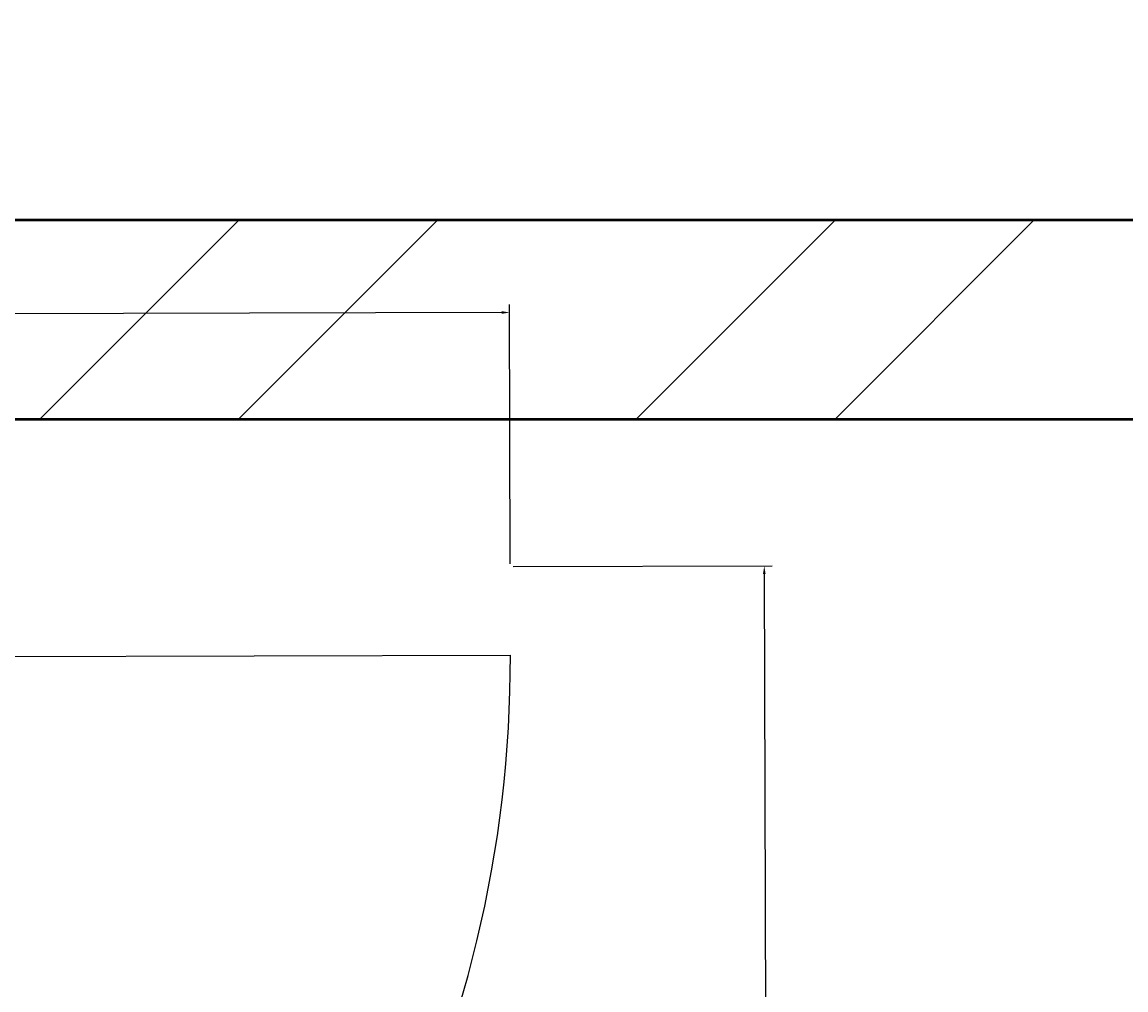
# Model space of a CAD drawing. Units: inches. Extents: x 963 to 2075, y 289 to 2657.
# Tile 11 of 98: x 1399 to 1424, y 1696 to 1718. Entities that reach past the tile are written whole.
import ezdxf

# ---------------------------------------------------------------- set-up
doc = ezdxf.new("R2010")
doc.units = ezdxf.units.IN
for name, color, linetype, lineweight in [('A-ANNO-DIMS', 2, 'Continuous', 18), ('A-DOOR', 4, 'Continuous', 25), ('A-WALL', 7, 'Continuous', 50), ('A-WALL-PATT', 8, 'Continuous', 13)]:
    doc.layers.add(name, color=color, linetype=linetype, lineweight=lineweight)
doc.styles.get("Standard").update_dxf_attribs({"font": 'arial.ttf'})
doc.dimstyles.get("Standard").update_dxf_attribs({"dimtxt": 0.18, "dimasz": 0.18, "dimexe": 0.18, "dimexo": 0.0625, "dimgap": 0.09, "dimtad": 0, "dimtih": 1, "dimtoh": 1, "dimdec": 4, "dimzin": 0, "dimdsep": 46, "dimtxsty": 'Standard', "dimcen": 0.09, "dimadec": 0, "dimazin": 0, "dimtfac": 1, "dimtdec": 4, "dimtofl": 0, "dimtmove": 0, "dimatfit": 3, "dimfxl": 1, "dimtolj": 1, "dimtzin": 0, "dimarcsym": 0})

# ---------------------------------------------------------------- blocks, each defined once
blk = doc.blocks.new('DOOR-5')
blk.add_line((27.907, 36), (27.907, 0))
blk.add_arc((27.907, 27.321), 27.321, 161.4794, 270)
blk = doc.blocks.new('*D38')
at = {"layer": 'A-ANNO-DIMS', "color": 0, "lineweight": -2, "transparency": 16777216}
for p, q in [((1410.131, 1706.06), (1410.117, 1711.915)), ((1371.881, 1705.966), (1371.867, 1711.821)), ((1372.047, 1711.641), (1389.861, 1711.685)), ((1409.937, 1711.735), (1392.123, 1711.691))]:
    blk.add_line(p, q, dxfattribs=at)
at = {"layer": 'A-ANNO-DIMS', "color": 0, "transparency": 16777216}
for points in [[(1372.047, 1711.671), (1372.047, 1711.611), (1371.867, 1711.641)], [(1409.937, 1711.765), (1409.937, 1711.705), (1410.117, 1711.735)]]:
    blk.add_solid(points, dxfattribs=at)
at = {"layer": 'Defpoints', "color": 0, "transparency": 16777216}
for p in [(1371.867, 1711.641), (1410.131, 1705.998), (1371.881, 1705.903)]:
    blk.add_point(p, dxfattribs=at)
at = {"layer": 'A-ANNO-DIMS', "color": 0, "transparency": 16777216, "insert": (1390.992, 1711.688), "char_height": 0.18, "attachment_point": 5}
blk.add_mtext('\\A1;DOOR D5 38 TYP.', dxfattribs=at)
blk = doc.blocks.new('*D39')
at = {"layer": 'A-ANNO-DIMS', "color": 0, "lineweight": -2, "transparency": 16777216}
for p, q in [((1410.194, 1705.998), (1416.049, 1706.012)), ((1415.869, 1705.832), (1415.906, 1690.845)), ((1415.944, 1675.494), (1415.907, 1690.481)), ((1410.269, 1675.3), (1416.124, 1675.314))]:
    blk.add_line(p, q, dxfattribs=at)
at = {"layer": 'A-ANNO-DIMS', "color": 0, "transparency": 16777216}
for points in [[(1415.899, 1705.832), (1415.839, 1705.832), (1415.869, 1706.012)], [(1415.974, 1675.494), (1415.914, 1675.494), (1415.944, 1675.314)]]:
    blk.add_solid(points, dxfattribs=at)
at = {"layer": 'Defpoints', "color": 0, "transparency": 16777216}
for p in [(1410.131, 1705.998), (1415.869, 1706.012), (1410.207, 1675.299)]:
    blk.add_point(p, dxfattribs=at)
at = {"layer": 'A-ANNO-DIMS', "color": 0, "transparency": 16777216, "insert": (1415.906, 1690.663), "char_height": 0.18, "attachment_point": 5}
blk.add_mtext('\\A1;31 TYP.', dxfattribs=at)

msp = doc.modelspace()

# ---------------------------------------------------------------- hatches: boundary and pattern name
at = {"layer": 'A-WALL-PATT'}
h = msp.add_hatch(dxfattribs=at)
h.set_pattern_fill('ANSI32', color=256)
h.paths.add_polyline_path([(1296.922, 2558.318), (1203.922, 2558.318), (1203.922, 2493.818), (1191.533, 2493.818), (1191.533, 2489.318), (1211.063, 2489.318), (1211.063, 2492.02), (1211.063, 2493.818), (1208.422, 2493.818), (1208.422, 2553.818), (1292.422, 2553.818), (1292.422, 2538.863), (1296.922, 2538.863)])
h.paths.add_polyline_path([(1442.422, 2558.318), (1349.422, 2558.318), (1349.422, 2538.943), (1353.922, 2538.943), (1353.922, 2553.818), (1437.922, 2553.818), (1437.922, 2493.818), (1434.542, 2493.818), (1434.542, 2489.318), (1448.311, 2489.318), (1448.311, 2491.568), (1448.311, 2493.818), (1442.422, 2493.818)])
h.paths.add_polyline_path([(1415.554, 2491.568), (1415.554, 2493.818), (1340.941, 2493.818), (1340.941, 2489.318), (1371.922, 2489.318), (1371.922, 2378.318), (1367.596, 2378.318), (1367.596, 2373.818), (1371.922, 2373.818), (1371.922, 2355.185), (1376.422, 2355.185), (1376.422, 2489.318), (1415.554, 2489.318)])
h.paths.add_polyline_path([(1304.941, 2491.568), (1304.941, 2493.818), (1296.922, 2493.818), (1296.922, 2514.863), (1292.422, 2514.863), (1292.422, 2493.818), (1232.808, 2493.818), (1232.808, 2489.318), (1256.422, 2489.318), (1256.422, 2327.318), (1253.714, 2327.318), (1253.714, 2322.818), (1328.422, 2322.818), (1328.422, 2331.147), (1323.922, 2331.147), (1323.922, 2327.318), (1260.922, 2327.318), (1260.922, 2373.818), (1323.922, 2373.818), (1323.922, 2357.812), (1328.422, 2357.812), (1328.422, 2373.818), (1346.007, 2373.818), (1346.007, 2376.068), (1346.007, 2378.318), (1260.922, 2378.318), (1260.922, 2489.318), (1304.941, 2489.318)])
h.paths.add_polyline_path([(1226.654, 2327.318), (1124.422, 2327.318), (1124.422, 2347.447), (1119.922, 2347.447), (1119.922, 2322.818), (1163.422, 2322.818), (1163.422, 2305.435), (1165.672, 2305.435), (1167.922, 2305.435), (1167.922, 2322.818), (1226.654, 2322.818), (1226.654, 2325.068)])
h.paths.add_polyline_path([(1095.922, 2489.318), (1124.422, 2489.318), (1131.533, 2489.318), (1131.533, 2491.568), (1131.533, 2493.818), (1119.922, 2493.818), (1091.422, 2493.818), (1091.422, 2417.318), (1095.922, 2417.318), (1119.922, 2417.318), (1119.922, 2407.447), (1124.422, 2407.447), (1124.422, 2421.818), (1095.922, 2421.818)])
h.paths.add_polyline_path([(1512.922, 2558.318), (1508.422, 2558.318), (1508.422, 2493.818), (1503.401, 2493.818), (1503.401, 2489.318), (1508.422, 2489.318), (1508.422, 2327.318), (1376.422, 2327.318), (1376.422, 2330.273), (1371.922, 2330.273), (1371.922, 2298.744), (1376.422, 2298.744), (1376.422, 2322.818), (1508.422, 2322.818), (1508.422, 2165.318), (1504.255, 2165.318), (1504.255, 2160.818), (1508.422, 2160.818), (1508.422, 2108.318), (1512.922, 2108.318), (1512.922, 2160.818), (1516.182, 2160.818), (1516.182, 2163.068), (1516.182, 2165.318), (1512.922, 2165.318), (1512.922, 2322.818), (1644.922, 2322.818), (1644.922, 2298.744), (1649.422, 2298.744), (1649.422, 2322.818), (1649.422, 2330.944), (1647.172, 2330.944), (1644.922, 2330.944), (1644.922, 2327.318), (1512.922, 2327.318), (1512.922, 2489.318), (1516.759, 2489.318), (1516.759, 2491.568), (1516.759, 2493.818), (1512.922, 2493.818)])
h.paths.add_polyline_path([(1671.922, 2558.318), (1578.922, 2558.318), (1578.922, 2493.818), (1573.526, 2493.818), (1573.526, 2489.318), (1586.537, 2489.318), (1586.537, 2491.568), (1586.537, 2493.818), (1583.422, 2493.818), (1583.422, 2553.818), (1667.422, 2553.818), (1667.422, 2541.109), (1671.922, 2541.109)])
h.paths.add_polyline_path([(1681.257, 2493.818), (1671.922, 2493.818), (1671.922, 2517.109), (1667.422, 2517.109), (1667.422, 2493.818), (1610.218, 2493.818), (1610.218, 2489.318), (1644.922, 2489.318), (1644.922, 2357.865), (1649.422, 2357.865), (1649.422, 2373.818), (1652.203, 2373.818), (1652.203, 2375.827), (1652.203, 2378.318), (1649.422, 2378.318), (1649.422, 2489.318), (1681.257, 2489.318), (1681.257, 2491.568)])
h.paths.add_polyline_path([(1821.922, 2558.318), (1728.922, 2558.318), (1728.922, 2541), (1733.422, 2541), (1733.422, 2553.818), (1817.422, 2553.818), (1817.422, 2493.818), (1813.507, 2493.818), (1813.507, 2489.318), (1830.078, 2489.318), (1830.078, 2491.568), (1830.078, 2493.818), (1821.922, 2493.818)])
h.paths.add_polyline_path([(1794.244, 2493.818), (1717.257, 2493.818), (1717.257, 2489.318), (1760.422, 2489.318), (1760.422, 2378.318), (1674.401, 2378.318), (1674.401, 2373.818), (1692.922, 2373.818), (1692.922, 2356.954), (1697.422, 2356.954), (1697.422, 2373.818), (1760.422, 2373.818), (1760.422, 2327.318), (1697.422, 2327.318), (1697.422, 2333.341), (1692.922, 2333.341), (1692.922, 2322.818), (1768.037, 2322.818), (1768.037, 2325.068), (1768.037, 2327.318), (1764.922, 2327.318), (1764.922, 2489.318), (1794.244, 2489.318)])
h.paths.add_polyline_path([(1733.422, 2517), (1728.922, 2517), (1728.922, 2493.818), (1733.422, 2493.818)], flags=17)
h.paths.add_polyline_path([(1929.922, 2493.818), (1890.078, 2493.818), (1890.078, 2489.318), (1896.922, 2489.318), (1925.422, 2489.318), (1925.422, 2421.818), (1896.922, 2421.818), (1896.922, 2408.318), (1901.422, 2408.318), (1901.422, 2417.318), (1925.422, 2417.318), (1929.922, 2417.318)])
h.paths.add_polyline_path([(1901.422, 2348.318), (1896.922, 2348.318), (1896.922, 2327.318), (1800.423, 2327.318), (1800.423, 2322.818), (1853.422, 2322.818), (1853.422, 2309.453), (1857.922, 2309.453), (1857.922, 2322.818), (1901.422, 2322.818)])
h.paths.add_polyline_path([(1857.922, 2249.453), (1853.422, 2249.453), (1853.422, 2214.818), (1686.309, 2214.818), (1686.309, 2210.318), (1853.422, 2210.318), (1853.422, 2202.134), (1857.922, 2202.134), (1857.922, 2210.318)])
h.paths.add_polyline_path([(1857.922, 2142.134), (1853.422, 2142.134), (1853.422, 2115.422), (1841.422, 2115.422), (1841.422, 2088.531), (1841.422, 2046.949), (1845.922, 2046.949), (1845.922, 2110.922), (1905.922, 2110.922), (1905.922, 2092.517), (1910.422, 2092.517), (1910.422, 2115.422), (1857.922, 2115.422)])
h.paths.add_polyline_path([(1532.436, 1482.342), (1573.456, 1482.342), (1573.456, 1501), (1532.436, 1501)], flags=9)
h.paths.add_polyline_path([(1438.658, 1486.302), (1479.678, 1486.302), (1479.678, 1504.96), (1438.658, 1504.96)], flags=9)
h.paths.add_polyline_path([(1411.215, 1365.308), (1659.139, 1365.308), (1659.139, 1402.401), (1411.215, 1402.401)], flags=9)
h.paths.add_polyline_path([(1185.671, 2296.298), (1248.16, 2296.298), (1248.16, 2314.955), (1185.671, 2314.955)], flags=9)
h.paths.add_polyline_path([(1177.31, 2187.35), (1216.15, 2187.35), (1216.15, 2206.007), (1177.31, 2206.007)], flags=9)
h.paths.add_polyline_path([(1295.101, 1602.083), (1328.26, 1602.083), (1328.26, 1620.741), (1295.101, 1620.741)], flags=9)
h.paths.add_polyline_path([(1525.126, 2005.99), (1558.39, 2005.99), (1558.39, 2024.648), (1525.126, 2024.648)], flags=9)
h.paths.add_polyline_path([(1459.606, 1977.125), (1472.195, 1977.125), (1472.195, 1987.429), (1459.606, 1987.429)], flags=9)
h.paths.add_polyline_path([(1467.815, 2053.676), (1480.018, 2053.676), (1480.018, 2063.979), (1467.815, 2063.979)], flags=9)
h.paths.add_polyline_path([(1555.184, 2119.02), (1584.563, 2119.02), (1584.563, 2137.678), (1555.184, 2137.678)], flags=25)
h.paths.add_polyline_path([(1405.389, 2115.291), (1444.478, 2115.291), (1444.478, 2133.948), (1405.389, 2133.948)], flags=25)
h.paths.add_polyline_path([(1698.482, 2004.259), (1727.695, 2004.259), (1727.695, 2022.916), (1698.482, 2022.916)], flags=9)
h.paths.add_polyline_path([(1612.158, 1972.855), (1629.016, 1972.855), (1629.016, 1983.159), (1612.158, 1983.159)], flags=9)
h.paths.add_polyline_path([(1608.289, 2060.036), (1625.147, 2060.036), (1625.147, 2070.34), (1608.289, 2070.34)], flags=9)
h.paths.add_polyline_path([(1527.954, 1684.402), (1566.795, 1684.402), (1566.795, 1703.06), (1527.954, 1703.06)], flags=9)
h.paths.add_polyline_path([(1422.792, 1683.59), (1461.633, 1683.59), (1461.633, 1702.247), (1422.792, 1702.247)], flags=9)
h.paths.add_polyline_path([(1531.262, 1732.459), (1574.015, 1732.459), (1574.015, 1751.116), (1531.262, 1751.116)], flags=9)
h.paths.add_polyline_path([(1402.872, 1732.845), (1439.799, 1732.845), (1439.799, 1751.502), (1402.872, 1751.502)], flags=9)
h.paths.add_polyline_path([(1243.122, 1923.132), (1281.962, 1923.132), (1281.962, 1941.79), (1243.122, 1941.79)], flags=9)
h.paths.add_polyline_path([(1181.752, 1792.268), (1244.241, 1792.268), (1244.241, 1810.926), (1181.752, 1810.926)], flags=9)
h.paths.add_polyline_path([(1265.822, 1670.3), (1316.071, 1670.3), (1316.071, 1688.957), (1265.822, 1688.957)], flags=9)
h.paths.add_polyline_path([(1140.263, 1676.054), (1179.104, 1676.054), (1179.104, 1694.711), (1140.263, 1694.711)], flags=9)
h.paths.add_polyline_path([(1107.49, 1490.889), (1143.374, 1490.889), (1143.374, 1509.546), (1107.49, 1509.546)], flags=9)
h.paths.add_polyline_path([(1217.584, 1483.899), (1246.741, 1483.899), (1246.741, 1502.556), (1217.584, 1502.556)], flags=9)
h.paths.add_polyline_path([(1389.21, 1486.919), (1418.367, 1486.919), (1418.367, 1505.576), (1389.21, 1505.576)], flags=9)
h.paths.add_polyline_path([(1672.208, 1602.083), (1705.366, 1602.083), (1705.366, 1620.741), (1672.208, 1620.741)], flags=9)
h.paths.add_polyline_path([(1752.082, 1522.638), (1781.24, 1522.638), (1781.24, 1541.295), (1752.082, 1541.295)], flags=9)
h.paths.add_polyline_path([(1848.275, 1491.26), (1884.158, 1491.26), (1884.158, 1509.918), (1848.275, 1509.918)], flags=9)
h.paths.add_polyline_path([(1822.47, 1685.62), (1861.31, 1685.62), (1861.31, 1704.278), (1822.47, 1704.278)], flags=9)
h.paths.add_polyline_path([(1713.195, 1672.232), (1763.444, 1672.232), (1763.444, 1690.889), (1713.195, 1690.889)], flags=9)
h.paths.add_polyline_path([(1736.619, 1790.578), (1799.109, 1790.578), (1799.109, 1809.235), (1736.619, 1809.235)], flags=9)
h.paths.add_polyline_path([(1691.491, 1916.355), (1730.332, 1916.355), (1730.332, 1935.013), (1691.491, 1935.013)], flags=9)
h.paths.add_polyline_path([(1764.872, 1973.922), (1794.306, 1973.922), (1794.306, 1992.58), (1764.872, 1992.58)], flags=9)
h.paths.add_polyline_path([(1767.854, 2034.017), (1797.288, 2034.017), (1797.288, 2052.674), (1767.854, 2052.674)], flags=9)
h.paths.add_polyline_path([(1851.593, 2060.331), (1880.751, 2060.331), (1880.751, 2078.989), (1851.593, 2078.989)], flags=25)
h.paths.add_polyline_path([(1688.491, 2086.874), (1727.332, 2086.874), (1727.332, 2105.531), (1688.491, 2105.531)], flags=9)
h.paths.add_polyline_path([(1537.743, 2293.581), (1580.495, 2293.581), (1580.495, 2312.239), (1537.743, 2312.239)], flags=25)
h.paths.add_polyline_path([(1425.587, 2296.109), (1468.34, 2296.109), (1468.34, 2314.766), (1425.587, 2314.766)], flags=25)
h.paths.add_polyline_path([(1278.518, 2004.184), (1307.72, 2004.184), (1307.72, 2022.841), (1278.518, 2022.841)], flags=9)
h.paths.add_polyline_path([(1193.282, 1973.635), (1222.715, 1973.635), (1222.715, 1992.292), (1193.282, 1992.292)], flags=9)
h.paths.add_polyline_path([(1192.411, 2040.577), (1221.845, 2040.577), (1221.845, 2059.234), (1192.411, 2059.234)], flags=9)
h.paths.add_polyline_path([(1130.603, 1951.393), (1159.76, 1951.393), (1159.76, 1970.05), (1130.603, 1970.05)], flags=9)
h.paths.add_polyline_path([(1132.827, 2052.494), (1161.984, 2052.494), (1161.984, 2071.151), (1132.827, 2071.151)], flags=9)
h.paths.add_polyline_path([(1265.128, 2334.619), (1315.377, 2334.619), (1315.377, 2353.277), (1265.128, 2353.277)], flags=25)
h.paths.add_polyline_path([(1136.741, 2330.785), (1175.582, 2330.785), (1175.582, 2349.443), (1136.741, 2349.443)], flags=9)
h.paths.add_polyline_path([(1287.422, 2417.204), (1320.58, 2417.204), (1320.58, 2435.861), (1287.422, 2435.861)], flags=25)
h.paths.add_polyline_path([(1430.988, 2329.159), (1469.828, 2329.159), (1469.828, 2347.816), (1430.988, 2347.816)], flags=25)
h.paths.add_polyline_path([(1525.424, 2329.213), (1564.264, 2329.213), (1564.264, 2347.87), (1525.424, 2347.87)], flags=25)
h.paths.add_polyline_path([(1684.525, 2382.799), (1717.683, 2382.799), (1717.683, 2401.457), (1684.525, 2401.457)], flags=25)
h.paths.add_polyline_path([(1704.805, 2340.293), (1755.054, 2340.293), (1755.054, 2358.95), (1704.805, 2358.95)], flags=25)
h.paths.add_polyline_path([(1694.113, 2287.757), (1756.602, 2287.757), (1756.602, 2306.414), (1694.113, 2306.414)], flags=9)
h.paths.add_polyline_path([(1815.778, 2329.861), (1854.618, 2329.861), (1854.618, 2348.518), (1815.778, 2348.518)], flags=9)
h.paths.add_polyline_path([(1842.873, 2514.256), (1878.756, 2514.256), (1878.756, 2532.914), (1842.873, 2532.914)], flags=9)
h.paths.add_polyline_path([(1769.513, 2531.447), (1798.671, 2531.447), (1798.671, 2550.104), (1769.513, 2550.104)], flags=25)
h.paths.add_polyline_path([(1594.772, 2518.468), (1623.93, 2518.468), (1623.93, 2537.125), (1594.772, 2537.125)], flags=25)
h.paths.add_polyline_path([(1520.723, 2516.185), (1556.606, 2516.185), (1556.606, 2534.842), (1520.723, 2534.842)], flags=25)
h.paths.add_polyline_path([(1464.456, 2516.694), (1500.34, 2516.694), (1500.34, 2535.351), (1464.456, 2535.351)], flags=25)
h.paths.add_polyline_path([(1365.696, 2528.97), (1394.854, 2528.97), (1394.854, 2547.627), (1365.696, 2547.627)], flags=25)
h.paths.add_polyline_path([(1222.838, 2516.231), (1251.995, 2516.231), (1251.995, 2534.889), (1222.838, 2534.889)], flags=25)
h.paths.add_polyline_path([(1104.545, 2509.6), (1140.429, 2509.6), (1140.429, 2528.257), (1104.545, 2528.257)], flags=9)
h = msp.add_hatch(dxfattribs=at)
h.set_pattern_fill('ANSI32', color=256)
h.paths.add_polyline_path([(1335.968, 2212.568), (1335.968, 2214.818), (1167.922, 2214.818), (1167.922, 2245.435), (1163.422, 2245.435), (1163.422, 2210.318), (1163.422, 2194.812), (1167.922, 2194.812), (1167.922, 2210.318), (1335.968, 2210.318)])
h.paths.add_polyline_path([(1532.436, 1482.342), (1573.456, 1482.342), (1573.456, 1501), (1532.436, 1501)], flags=9)
h.paths.add_polyline_path([(1438.658, 1486.302), (1479.678, 1486.302), (1479.678, 1504.96), (1438.658, 1504.96)], flags=9)
h.paths.add_polyline_path([(1411.215, 1365.308), (1659.139, 1365.308), (1659.139, 1402.401), (1411.215, 1402.401)], flags=9)
h.paths.add_polyline_path([(1185.671, 2296.298), (1248.16, 2296.298), (1248.16, 2314.955), (1185.671, 2314.955)], flags=9)
h.paths.add_polyline_path([(1177.31, 2187.35), (1216.15, 2187.35), (1216.15, 2206.007), (1177.31, 2206.007)], flags=9)
h.paths.add_polyline_path([(1295.101, 1602.083), (1328.26, 1602.083), (1328.26, 1620.741), (1295.101, 1620.741)], flags=9)
h.paths.add_polyline_path([(1525.126, 2005.99), (1558.39, 2005.99), (1558.39, 2024.648), (1525.126, 2024.648)], flags=9)
h.paths.add_polyline_path([(1459.606, 1977.125), (1472.195, 1977.125), (1472.195, 1987.429), (1459.606, 1987.429)], flags=9)
h.paths.add_polyline_path([(1467.815, 2053.676), (1480.018, 2053.676), (1480.018, 2063.979), (1467.815, 2063.979)], flags=9)
h.paths.add_polyline_path([(1555.184, 2119.02), (1584.563, 2119.02), (1584.563, 2137.678), (1555.184, 2137.678)], flags=9)
h.paths.add_polyline_path([(1405.389, 2115.291), (1444.478, 2115.291), (1444.478, 2133.948), (1405.389, 2133.948)], flags=9)
h.paths.add_polyline_path([(1698.482, 2004.259), (1727.695, 2004.259), (1727.695, 2022.916), (1698.482, 2022.916)], flags=9)
h.paths.add_polyline_path([(1612.158, 1972.855), (1629.016, 1972.855), (1629.016, 1983.159), (1612.158, 1983.159)], flags=9)
h.paths.add_polyline_path([(1608.289, 2060.036), (1625.147, 2060.036), (1625.147, 2070.34), (1608.289, 2070.34)], flags=9)
h.paths.add_polyline_path([(1527.954, 1684.402), (1566.795, 1684.402), (1566.795, 1703.06), (1527.954, 1703.06)], flags=9)
h.paths.add_polyline_path([(1422.792, 1683.59), (1461.633, 1683.59), (1461.633, 1702.247), (1422.792, 1702.247)], flags=9)
h.paths.add_polyline_path([(1531.262, 1732.459), (1574.015, 1732.459), (1574.015, 1751.116), (1531.262, 1751.116)], flags=9)
h.paths.add_polyline_path([(1402.872, 1732.845), (1439.799, 1732.845), (1439.799, 1751.502), (1402.872, 1751.502)], flags=9)
h.paths.add_polyline_path([(1243.122, 1923.132), (1281.962, 1923.132), (1281.962, 1941.79), (1243.122, 1941.79)], flags=9)
h.paths.add_polyline_path([(1181.752, 1792.268), (1244.241, 1792.268), (1244.241, 1810.926), (1181.752, 1810.926)], flags=9)
h.paths.add_polyline_path([(1265.822, 1670.3), (1316.071, 1670.3), (1316.071, 1688.957), (1265.822, 1688.957)], flags=9)
h.paths.add_polyline_path([(1140.263, 1676.054), (1179.104, 1676.054), (1179.104, 1694.711), (1140.263, 1694.711)], flags=9)
h.paths.add_polyline_path([(1107.49, 1490.889), (1143.374, 1490.889), (1143.374, 1509.546), (1107.49, 1509.546)], flags=9)
h.paths.add_polyline_path([(1217.584, 1483.899), (1246.741, 1483.899), (1246.741, 1502.556), (1217.584, 1502.556)], flags=9)
h.paths.add_polyline_path([(1389.21, 1486.919), (1418.367, 1486.919), (1418.367, 1505.576), (1389.21, 1505.576)], flags=9)
h.paths.add_polyline_path([(1672.208, 1602.083), (1705.366, 1602.083), (1705.366, 1620.741), (1672.208, 1620.741)], flags=9)
h.paths.add_polyline_path([(1752.082, 1522.638), (1781.24, 1522.638), (1781.24, 1541.295), (1752.082, 1541.295)], flags=9)
h.paths.add_polyline_path([(1848.275, 1491.26), (1884.158, 1491.26), (1884.158, 1509.918), (1848.275, 1509.918)], flags=9)
h.paths.add_polyline_path([(1822.47, 1685.62), (1861.31, 1685.62), (1861.31, 1704.278), (1822.47, 1704.278)], flags=9)
h.paths.add_polyline_path([(1713.195, 1672.232), (1763.444, 1672.232), (1763.444, 1690.889), (1713.195, 1690.889)], flags=9)
h.paths.add_polyline_path([(1736.619, 1790.578), (1799.109, 1790.578), (1799.109, 1809.235), (1736.619, 1809.235)], flags=9)
h.paths.add_polyline_path([(1691.491, 1916.355), (1730.332, 1916.355), (1730.332, 1935.013), (1691.491, 1935.013)], flags=9)
h.paths.add_polyline_path([(1764.872, 1973.922), (1794.306, 1973.922), (1794.306, 1992.58), (1764.872, 1992.58)], flags=9)
h.paths.add_polyline_path([(1767.854, 2034.017), (1797.288, 2034.017), (1797.288, 2052.674), (1767.854, 2052.674)], flags=9)
h.paths.add_polyline_path([(1851.593, 2060.331), (1880.751, 2060.331), (1880.751, 2078.989), (1851.593, 2078.989)], flags=9)
h.paths.add_polyline_path([(1688.491, 2086.874), (1727.332, 2086.874), (1727.332, 2105.531), (1688.491, 2105.531)], flags=9)
h.paths.add_polyline_path([(1537.743, 2293.581), (1580.495, 2293.581), (1580.495, 2312.239), (1537.743, 2312.239)], flags=9)
h.paths.add_polyline_path([(1425.587, 2296.109), (1468.34, 2296.109), (1468.34, 2314.766), (1425.587, 2314.766)], flags=9)
h.paths.add_polyline_path([(1278.518, 2004.184), (1307.72, 2004.184), (1307.72, 2022.841), (1278.518, 2022.841)], flags=9)
h.paths.add_polyline_path([(1193.282, 1973.635), (1222.715, 1973.635), (1222.715, 1992.292), (1193.282, 1992.292)], flags=9)
h.paths.add_polyline_path([(1192.411, 2040.577), (1221.845, 2040.577), (1221.845, 2059.234), (1192.411, 2059.234)], flags=9)
h.paths.add_polyline_path([(1130.603, 1951.393), (1159.76, 1951.393), (1159.76, 1970.05), (1130.603, 1970.05)], flags=9)
h.paths.add_polyline_path([(1132.827, 2052.494), (1161.984, 2052.494), (1161.984, 2071.151), (1132.827, 2071.151)], flags=9)
h.paths.add_polyline_path([(1265.128, 2334.619), (1315.377, 2334.619), (1315.377, 2353.277), (1265.128, 2353.277)], flags=9)
h.paths.add_polyline_path([(1136.741, 2330.785), (1175.582, 2330.785), (1175.582, 2349.443), (1136.741, 2349.443)], flags=9)
h.paths.add_polyline_path([(1287.422, 2417.204), (1320.58, 2417.204), (1320.58, 2435.861), (1287.422, 2435.861)], flags=9)
h.paths.add_polyline_path([(1430.988, 2329.159), (1469.828, 2329.159), (1469.828, 2347.816), (1430.988, 2347.816)], flags=9)
h.paths.add_polyline_path([(1525.424, 2329.213), (1564.264, 2329.213), (1564.264, 2347.87), (1525.424, 2347.87)], flags=9)
h.paths.add_polyline_path([(1684.525, 2382.799), (1717.683, 2382.799), (1717.683, 2401.457), (1684.525, 2401.457)], flags=9)
h.paths.add_polyline_path([(1704.805, 2340.293), (1755.054, 2340.293), (1755.054, 2358.95), (1704.805, 2358.95)], flags=9)
h.paths.add_polyline_path([(1694.113, 2287.757), (1756.602, 2287.757), (1756.602, 2306.414), (1694.113, 2306.414)], flags=9)
h.paths.add_polyline_path([(1815.778, 2329.861), (1854.618, 2329.861), (1854.618, 2348.518), (1815.778, 2348.518)], flags=9)
h.paths.add_polyline_path([(1842.873, 2514.256), (1878.756, 2514.256), (1878.756, 2532.914), (1842.873, 2532.914)], flags=9)
h.paths.add_polyline_path([(1769.513, 2531.447), (1798.671, 2531.447), (1798.671, 2550.104), (1769.513, 2550.104)], flags=9)
h.paths.add_polyline_path([(1594.772, 2518.468), (1623.93, 2518.468), (1623.93, 2537.125), (1594.772, 2537.125)], flags=9)
h.paths.add_polyline_path([(1520.723, 2516.185), (1556.606, 2516.185), (1556.606, 2534.842), (1520.723, 2534.842)], flags=9)
h.paths.add_polyline_path([(1464.456, 2516.694), (1500.34, 2516.694), (1500.34, 2535.351), (1464.456, 2535.351)], flags=9)
h.paths.add_polyline_path([(1365.696, 2528.97), (1394.854, 2528.97), (1394.854, 2547.627), (1365.696, 2547.627)], flags=9)
h.paths.add_polyline_path([(1222.838, 2516.231), (1251.995, 2516.231), (1251.995, 2534.889), (1222.838, 2534.889)], flags=9)
h.paths.add_polyline_path([(1104.545, 2509.6), (1140.429, 2509.6), (1140.429, 2528.257), (1104.545, 2528.257)], flags=9)
h = msp.add_hatch(dxfattribs=at)
h.set_pattern_fill('ANSI32', color=256)
h.paths.add_polyline_path([(1473.609, 2163.068), (1473.609, 2165.318), (1376.422, 2165.318), (1376.422, 2227.983), (1371.922, 2227.983), (1371.922, 2214.818), (1368.405, 2214.818), (1368.405, 2210.318), (1371.922, 2210.318), (1371.922, 2160.818), (1395.922, 2160.818), (1395.922, 2090.318), (1217.345, 2090.318), (1217.345, 2085.818), (1395.922, 2085.818), (1458.922, 2085.818), (1458.922, 2108.318), (1454.422, 2108.318), (1454.422, 2090.318), (1400.422, 2090.318), (1400.422, 2160.818), (1473.609, 2160.818)])
h.paths.add_polyline_path([(1649.422, 2210.318), (1653.225, 2210.318), (1653.225, 2214.818), (1649.422, 2214.818), (1649.422, 2227.983), (1644.922, 2227.983), (1644.922, 2165.318), (1550.099, 2165.318), (1550.099, 2160.818), (1620.922, 2160.818), (1620.922, 2112.818), (1555.446, 2112.818), (1555.446, 2108.318), (1584.327, 2108.318), (1584.327, 2084.916), (1588.827, 2084.916), (1588.827, 2108.318), (1625.422, 2108.318), (1667.951, 2108.318), (1667.951, 2022.667), (1588.827, 2022.667), (1588.827, 2047.408), (1584.327, 2047.408), (1584.327, 1996.003), (1588.827, 1996.003), (1588.827, 2018.318), (1667.951, 2018.167), (1667.951, 1928.318), (1625.422, 1928.318), (1625.422, 1923.818), (1672.451, 1923.818), (1672.451, 1928.318), (1672.451, 1946.663), (1785.446, 1946.663), (1785.446, 1951.163), (1743.034, 1951.163), (1743.034, 2017.922), (1841.422, 2017.922), (1841.422, 2014.775), (1845.922, 2014.775), (1845.922, 2017.922), (1905.922, 2017.922), (1905.922, 1987.511), (1910.422, 1987.511), (1910.422, 2022.422), (1910.422, 2068.517), (1905.922, 2068.517), (1905.922, 2022.422), (1845.922, 2022.422), (1845.922, 2025.851), (1843.672, 2025.851), (1841.422, 2025.851), (1841.422, 2022.422), (1743.034, 2022.422), (1743.034, 2084.031), (1768.451, 2084.031), (1785.446, 2084.031), (1785.446, 2088.531), (1672.451, 2088.531), (1672.451, 2112.818), (1667.951, 2112.818), (1625.422, 2112.818), (1625.422, 2160.818), (1649.422, 2160.818)])
h.paths.add_polyline_path([(1672.451, 2084.031), (1738.534, 2084.031), (1738.534, 1951.163), (1672.451, 1951.163)], flags=16)
h.paths.add_polyline_path([(1672.451, 2084.031), (1738.534, 2084.031), (1705.492, 2017.597)], flags=0)
h.paths.add_polyline_path([(1262.766, 2085.818), (1258.266, 2085.818), (1258.266, 2023.278), (1184.422, 2023.278), (1184.422, 2018.778), (1258.266, 2018.778), (1258.266, 1950.818), (1262.766, 1950.818)])
h.paths.add_polyline_path([(1312.266, 2085.818), (1307.766, 2085.818), (1307.766, 1950.818), (1312.266, 1950.818)])
h.paths.add_polyline_path([(1458.922, 1950.818), (1395.922, 1950.818), (1216.568, 1950.818), (1216.568, 1946.318), (1346.422, 1946.318), (1395.922, 1946.318), (1395.922, 1875.818), (1371.922, 1875.818), (1371.922, 1826.318), (1368.931, 1826.318), (1368.931, 1821.818), (1371.922, 1821.818), (1371.922, 1813.622), (1376.422, 1813.622), (1376.422, 1871.318), (1474.504, 1871.318), (1474.504, 1873.568), (1474.504, 1875.818), (1400.422, 1875.818), (1400.422, 1946.318), (1454.422, 1946.318), (1454.422, 1928.318), (1458.922, 1928.318)])
h.paths.add_polyline_path([(1184.422, 2120.778), (1167.922, 2120.778), (1167.922, 2134.812), (1165.672, 2134.812), (1163.422, 2134.812), (1163.422, 2120.778), (1119.922, 2120.778), (1119.922, 2098.095), (1124.422, 2098.095), (1124.422, 2116.278), (1167.922, 2116.278), (1179.922, 2116.278), (1179.922, 2045.916), (1184.422, 2045.916), (1184.422, 2090.318), (1184.422, 2116.278)])
h.paths.add_polyline_path([(1124.422, 2018.778), (1179.922, 2018.778), (1179.922, 2016.294), (1184.422, 2016.294), (1184.422, 2023.278), (1184.422, 2026.588), (1182.172, 2026.588), (1179.922, 2026.588), (1179.922, 2023.278), (1124.422, 2023.278), (1124.422, 2074.095), (1119.922, 2074.095), (1119.922, 2018.778), (1119.922, 1979.633), (1124.422, 1979.633)])
h.paths.add_polyline_path([(1184.422, 1925.778), (1184.422, 1946.318), (1184.422, 1996.073), (1182.172, 1996.073), (1179.922, 1996.073), (1179.922, 1925.778), (1124.422, 1925.778), (1124.422, 1955.633), (1119.922, 1955.502), (1119.922, 1921.278), (1158.922, 1921.278), (1158.922, 1909.983), (1163.422, 1909.983), (1163.422, 1921.278), (1184.422, 1921.278)])
h.paths.add_polyline_path([(1341.449, 1826.318), (1163.422, 1826.318), (1163.422, 1849.983), (1158.922, 1849.983), (1158.922, 1821.818), (1158.922, 1804.033), (1163.422, 1804.033), (1163.422, 1821.818), (1341.449, 1821.818)])
h.paths.add_polyline_path([(1222.981, 1713.818), (1163.422, 1713.818), (1163.422, 1744.033), (1161.172, 1744.033), (1158.922, 1744.033), (1158.922, 1713.818), (1119.922, 1713.818), (1119.922, 1694.65), (1124.422, 1694.65), (1124.422, 1709.318), (1158.922, 1709.318), (1222.981, 1709.318)])
h.paths.add_polyline_path([(1328.422, 1713.818), (1252.042, 1713.818), (1252.042, 1711.568), (1252.042, 1709.318), (1256.422, 1709.318), (1256.422, 1547.318), (1232.937, 1547.318), (1232.937, 1545.068), (1232.937, 1542.818), (1292.422, 1542.818), (1292.422, 1527.634), (1296.922, 1527.634), (1296.922, 1542.818), (1299.464, 1542.818), (1299.464, 1547.318), (1260.922, 1547.318), (1260.922, 1658.318), (1343.661, 1658.318), (1343.661, 1660.568), (1343.661, 1662.818), (1328.422, 1662.818), (1328.422, 1676.589), (1327.402, 1676.589), (1323.922, 1676.589), (1323.922, 1662.818), (1260.922, 1662.818), (1260.922, 1709.318), (1323.922, 1709.318), (1323.922, 1699.851), (1328.422, 1699.851)])
h.paths.add_polyline_path([(1649.422, 1875.818), (1625.422, 1875.818), (1625.422, 1928.318), (1620.922, 1928.318), (1588.827, 1928.318), (1588.827, 1950.59), (1584.327, 1950.59), (1584.327, 1928.318), (1555.446, 1928.318), (1555.446, 1923.818), (1620.922, 1923.818), (1620.922, 1875.818), (1548.952, 1875.818), (1548.952, 1873.568), (1548.952, 1871.318), (1644.922, 1871.318), (1644.922, 1813.622), (1649.422, 1813.622), (1649.422, 1821.818), (1652.045, 1821.818), (1652.045, 1824.068), (1652.045, 1826.318), (1649.422, 1826.318)])
h.paths.add_polyline_path([(1512.922, 1871.318), (1516.476, 1871.318), (1516.476, 1875.818), (1512.922, 1875.818), (1512.922, 1923.818), (1512.922, 1928.318), (1512.922, 1930.827), (1508.422, 1930.827), (1508.422, 1875.818), (1504.411, 1875.818), (1504.411, 1871.318), (1508.422, 1871.318), (1508.422, 1713.818), (1376.422, 1713.818), (1376.422, 1743.325), (1371.922, 1743.325), (1371.922, 1709.318), (1371.922, 1706.01), (1376.422, 1706.01), (1376.422, 1709.318), (1508.422, 1709.318), (1508.422, 1547.318), (1501.871, 1547.318), (1501.871, 1542.818), (1508.422, 1542.818), (1508.422, 1482.818), (1508.422, 1436.318), (1512.922, 1436.318), (1512.922, 1542.818), (1519.318, 1542.818), (1519.318, 1545.068), (1519.318, 1547.318), (1512.922, 1547.318), (1512.922, 1709.318), (1644.922, 1709.318), (1644.922, 1707.548), (1649.422, 1707.548), (1649.422, 1709.318), (1649.422, 1743.325), (1644.922, 1743.325), (1644.922, 1713.818), (1512.922, 1713.818)])
h.paths.add_polyline_path([(1129.884, 1545.068), (1129.884, 1547.318), (1124.422, 1547.318), (1095.922, 1547.318), (1095.922, 1614.818), (1124.422, 1614.818), (1124.422, 1619.318), (1095.922, 1619.318), (1091.422, 1619.318), (1091.422, 1542.818), (1095.922, 1542.818), (1119.922, 1542.818), (1129.884, 1542.818)])
h.paths.add_polyline_path([(1208.422, 1542.818), (1211.74, 1542.818), (1211.74, 1547.318), (1198.851, 1547.318), (1198.851, 1542.818), (1203.922, 1542.818), (1203.922, 1478.318), (1208.422, 1478.318), (1296.922, 1478.318), (1296.922, 1503.634), (1292.422, 1503.634), (1292.422, 1482.818), (1208.422, 1482.818)])
h.paths.add_polyline_path([(1430.422, 1542.818), (1435.699, 1542.818), (1435.699, 1545.068), (1435.699, 1547.318), (1422.658, 1547.318), (1422.658, 1545.068), (1422.658, 1542.818), (1425.922, 1542.818), (1425.922, 1482.857), (1341.922, 1482.857), (1341.922, 1502.732), (1337.422, 1502.732), (1337.422, 1478.357), (1425.922, 1478.357), (1425.922, 1440.818), (1425.922, 1436.318), (1430.422, 1436.318)])
h.paths.add_polyline_path([(1698.482, 2004.259), (1727.695, 2004.259), (1727.695, 2022.916), (1698.482, 2022.916)], flags=8)

# ---------------------------------------------------------------- linework, layer by layer
at = {"layer": 'A-WALL'}
for p, q in [((1508.422, 1713.818), (1376.422, 1713.818)), ((1508.422, 1709.318), (1376.422, 1709.318))]:
    msp.add_line(p, q, dxfattribs=at)

# ---------------------------------------------------------------- block references
at = {"layer": 'A-DOOR', "rotation": 90.14142652708767}
msp.add_blockref('DOOR-5', (1410.204, 1676.091), dxfattribs=at)

# ---------------------------------------------------------------- dimensions: what is measured, and where the dimension line sits
at = {"layer": 'A-ANNO-DIMS'}
for base, p1, p2, angle, text, picture, middle in [((1371.867, 1711.641), (1410.131, 1705.998), (1371.881, 1705.903), 180.1414, 'DOOR D5 <> TYP.', '*D38', (1390.992, 1711.688)), ((1415.869, 1706.012), (1410.207, 1675.299), (1410.131, 1705.998), 90.1414, '<> TYP.', '*D39', (1415.906, 1690.663))]:
    dim = msp.add_linear_dim(base=base, p1=p1, p2=p2, angle=angle, text=text, dimstyle='Standard', override={"dimdec": 0, "dimlfac": 1, "dimrnd": 0, "dimzin": 0, "dimdsep": 46, "dimlunit": 2}, dxfattribs=at)
    dim.commit()
    dim.dimension.update_dxf_attribs({"geometry": picture, "text_midpoint": middle})

doc.saveas('drawing.dxf')
